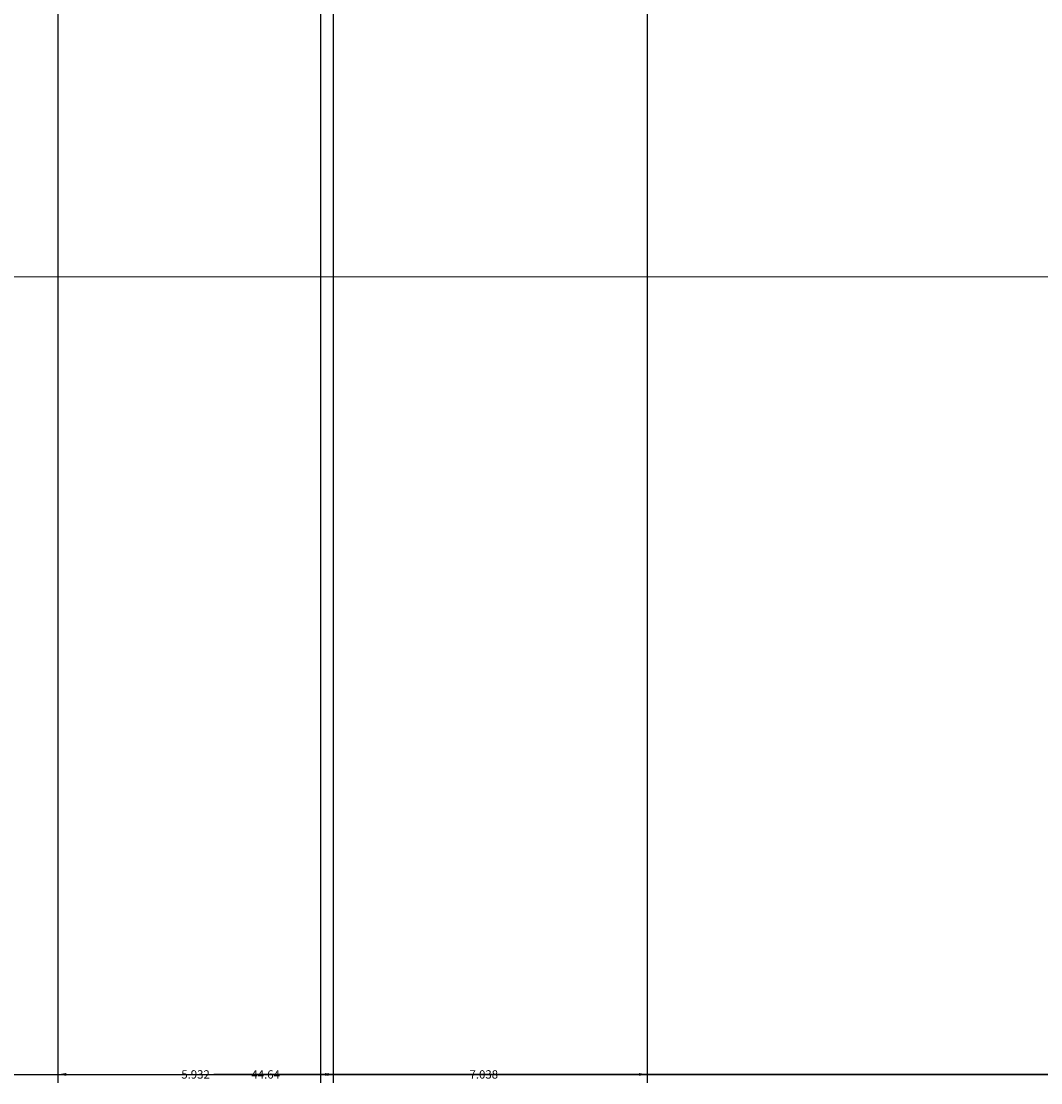
# Model space of a CAD drawing. Units: inches. Extents: x 412 to 584, y 208 to 437.
# Tile 3 of 28: x 472 to 494, y 208 to 231. Entities that reach past the tile are written whole.
import ezdxf

# ---------------------------------------------------------------- set-up
doc = ezdxf.new("R2010")
doc.units = ezdxf.units.IN
doc.header["$MEASUREMENT"] = 0
doc.layers.add('A-ANNO-DIMS', color=2, linetype='Continuous', lineweight=18)
doc.layers.add('E-ENCL', color=8, linetype='Continuous', lineweight=18)
doc.styles.get("Standard").update_dxf_attribs({"font": 'arial.ttf'})
doc.dimstyles.get("Standard").update_dxf_attribs({"dimtxt": 0.18, "dimasz": 0.18, "dimexe": 0.18, "dimexo": 0.0625, "dimgap": 0.09, "dimtad": 0, "dimtih": 1, "dimtoh": 1, "dimdec": 4, "dimzin": 0, "dimdsep": 46, "dimtxsty": 'Standard', "dimcen": 0.09, "dimadec": 0, "dimazin": 0, "dimtfac": 1, "dimtdec": 4, "dimtofl": 0, "dimtmove": 0, "dimatfit": 3, "dimfxl": 1, "dimtolj": 1, "dimtzin": 0, "dimarcsym": 0})

# ---------------------------------------------------------------- blocks, each defined once
blk = doc.blocks.new('*D13')
at = {"layer": 'A-ANNO-DIMS', "color": 0, "lineweight": -2, "transparency": 16777216}
for p, q in [((423.556, 225.526), (423.556, 208.233)), ((572.394, 225.526), (572.394, 208.233)), ((423.736, 208.413), (497.52, 208.413)), ((572.214, 208.413), (498.43, 208.413))]:
    blk.add_line(p, q, dxfattribs=at)
at = {"layer": 'A-ANNO-DIMS', "color": 0, "transparency": 16777216}
for points in [[(423.736, 208.443), (423.736, 208.383), (423.556, 208.413)], [(572.214, 208.443), (572.214, 208.383), (572.394, 208.413)]]:
    blk.add_solid(points, dxfattribs=at)
at = {"layer": 'Defpoints', "color": 0, "transparency": 16777216}
for p in [(423.556, 225.588), (572.394, 225.588), (572.394, 208.413)]:
    blk.add_point(p, dxfattribs=at)
at = {"layer": 'A-ANNO-DIMS', "color": 0, "transparency": 16777216, "insert": (497.975, 208.413), "char_height": 0.18, "attachment_point": 5}
blk.add_mtext('\\A1;148.84', dxfattribs=at)
blk = doc.blocks.new('*D15')
at = {"layer": 'A-ANNO-DIMS', "color": 0, "lineweight": -2, "transparency": 16777216}
for p, q in [((454.644, 219.451), (454.644, 208.233)), ((499.288, 219.47), (499.288, 208.233)), ((454.824, 208.413), (476.569, 208.413)), ((499.108, 208.413), (477.363, 208.413))]:
    blk.add_line(p, q, dxfattribs=at)
at = {"layer": 'A-ANNO-DIMS', "color": 0, "transparency": 16777216}
for points in [[(454.824, 208.443), (454.824, 208.383), (454.644, 208.413)], [(499.108, 208.443), (499.108, 208.383), (499.288, 208.413)]]:
    blk.add_solid(points, dxfattribs=at)
at = {"layer": 'Defpoints', "color": 0, "transparency": 16777216}
for p in [(454.644, 219.513), (499.288, 219.533), (499.288, 208.413)]:
    blk.add_point(p, dxfattribs=at)
at = {"layer": 'A-ANNO-DIMS', "color": 0, "transparency": 16777216, "insert": (476.966, 208.413), "char_height": 0.18, "attachment_point": 5}
blk.add_mtext('\\A1;44.64', dxfattribs=at)
blk = doc.blocks.new('*D33')
at = {"layer": 'A-ANNO-DIMS', "color": 0, "lineweight": -2, "transparency": 16777216}
for p, q in [((472.49, 363.226), (472.49, 208.233)), ((478.422, 363.226), (478.422, 208.233)), ((472.67, 208.413), (475.064, 208.413)), ((478.242, 208.413), (475.849, 208.413))]:
    blk.add_line(p, q, dxfattribs=at)
at = {"layer": 'A-ANNO-DIMS', "color": 0, "transparency": 16777216}
for points in [[(472.67, 208.443), (472.67, 208.383), (472.49, 208.413)], [(478.242, 208.443), (478.242, 208.383), (478.422, 208.413)]]:
    blk.add_solid(points, dxfattribs=at)
at = {"layer": 'Defpoints', "color": 0, "transparency": 16777216}
for p in [(472.49, 363.289), (478.422, 363.289), (478.422, 208.413)]:
    blk.add_point(p, dxfattribs=at)
at = {"layer": 'A-ANNO-DIMS', "color": 0, "transparency": 16777216, "insert": (475.456, 208.413), "char_height": 0.18, "attachment_point": 5}
blk.add_mtext('\\A1;5.932', dxfattribs=at)
blk = doc.blocks.new('*D34')
at = {"layer": 'A-ANNO-DIMS', "color": 0, "lineweight": -2, "transparency": 16777216}
for p, q in [((478.144, 276.254), (478.144, 208.233)), ((485.182, 276.254), (485.182, 208.233)), ((478.324, 208.413), (481.27, 208.413)), ((485.002, 208.413), (482.056, 208.413))]:
    blk.add_line(p, q, dxfattribs=at)
at = {"layer": 'A-ANNO-DIMS', "color": 0, "transparency": 16777216}
for points in [[(478.324, 208.443), (478.324, 208.383), (478.144, 208.413)], [(485.002, 208.443), (485.002, 208.383), (485.182, 208.413)]]:
    blk.add_solid(points, dxfattribs=at)
at = {"layer": 'Defpoints', "color": 0, "transparency": 16777216}
for p in [(478.144, 276.317), (485.182, 276.317), (485.182, 208.413)]:
    blk.add_point(p, dxfattribs=at)
at = {"layer": 'A-ANNO-DIMS', "color": 0, "transparency": 16777216, "insert": (481.663, 208.413), "char_height": 0.18, "attachment_point": 5}
blk.add_mtext('\\A1;7.038', dxfattribs=at)

msp = doc.modelspace()

# ---------------------------------------------------------------- linework, layer by layer
at = {"layer": 'E-ENCL'}
msp.add_lwpolyline([(423.5562, 309.3773), (572.3937, 309.3773), (572.3937, 225.5881), (423.5562, 225.5881)], close=True, dxfattribs=at)

# ---------------------------------------------------------------- dimensions: what is measured, and where the dimension line sits
at = {"layer": 'A-ANNO-DIMS'}
for base, p1, p2, override, picture, middle in [((478.4225, 208.4133), (472.4903, 363.2888), (478.4225, 363.2888), {"dimdec": 3, "dimlfac": 1, "dimrnd": 0, "dimzin": 0, "dimdsep": 46, "dimlunit": 2}, '*D33', (475.4564, 208.4133)), ((485.1817, 208.4133), (478.1437, 276.3167), (485.1817, 276.3167), {"dimdec": 3, "dimlfac": 1, "dimrnd": 0, "dimzin": 0, "dimdsep": 46, "dimlunit": 2}, '*D34', (481.6627, 208.4133)), ((572.3937, 208.4133), (423.5562, 225.5881), (572.3937, 225.5881), {"dimdec": 2, "dimlfac": 1, "dimrnd": 0, "dimzin": 0, "dimdsep": 46, "dimlunit": 2}, '*D13', (497.975, 208.4133)), ((499.2878, 208.4133), (454.6441, 219.5133), (499.2878, 219.5329), {"dimdec": 2, "dimlfac": 1, "dimrnd": 0, "dimzin": 0, "dimdsep": 46, "dimlunit": 2}, '*D15', (476.9659, 208.4133))]:
    dim = msp.add_linear_dim(base=base, p1=p1, p2=p2, dimstyle='Standard', override=override, dxfattribs=at)
    dim.commit()
    dim.dimension.update_dxf_attribs({"geometry": picture, "text_midpoint": middle})

doc.saveas('drawing.dxf')
